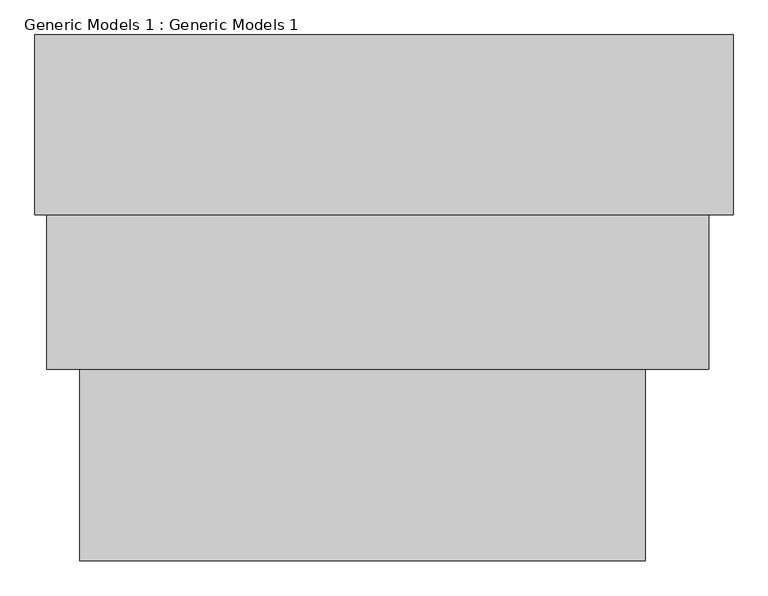
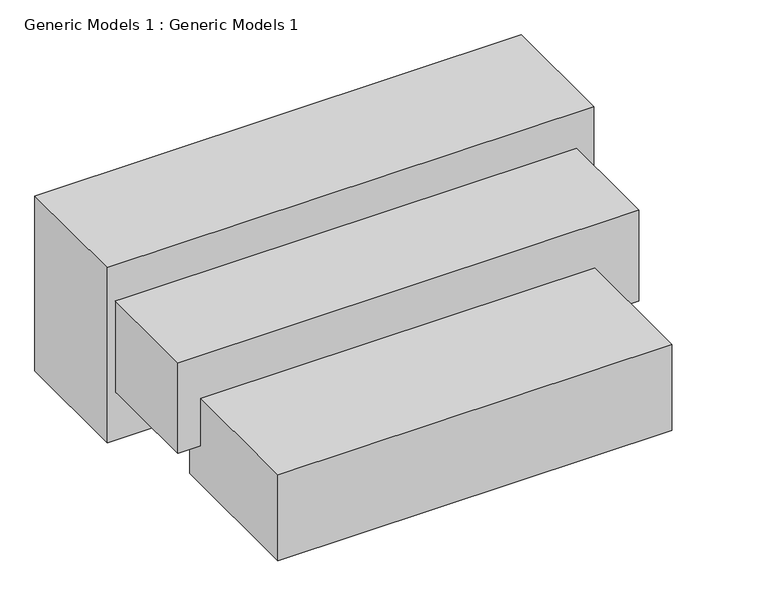
"""IFC4 building model written with IfcOpenShell, lengths in millimetres: proxy geometry, Generic Models 1 : Generic Models 1."""

from ifc_helpers import new_model, si_unit, frame, origin, place, context, project, spatial, polyline, outline, extrude, source, transform, mapped, element, save


def generic_models_1_generic_models_1_22b824c4(model_context):
    return source(origin(), model_context, "Body", "SweptSolid", [
        extrude(outline(polyline([(2976.4110568, 1086.8719151), (2976.4110568, 1471.821948), (3971.3936323, 1471.821948), (3971.3936323, 1086.8719151), (2976.4110568, 1086.8719151)])), frame((0.0, 0.0, -178.9427451), z_axis=(0.0, 0.0, 1.0), x_axis=(1.0, 0.0, 0.0)), (0.0, 0.0, 1.0), 229.7562689),
        extrude(outline(polyline([(2918.2285918, 1423.9390503), (2918.2285918, 1779.7588841), (4083.05, 1779.7588841), (4083.05, 1423.9390503), (2918.2285918, 1423.9390503)])), frame((0.0, 0.0, -76.2), z_axis=(0.0, 0.0, 1.0), x_axis=(1.0, 0.0, 0.0)), (0.0, 0.0, 1.0), 242.6189423),
        extrude(outline(polyline([(2897.395046, 1696.0473527), (2897.395046, 2012.5100722), (4126.0919946, 2012.5100722), (4126.0919946, 1696.0473527), (2897.395046, 1696.0473527)])), frame((0.0, 0.0, -204.7690848), z_axis=(0.0, 0.0, 1.0), x_axis=(1.0, 0.0, 0.0)), (0.0, 0.0, 1.0), 467.5207201),
    ])


if __name__ == "__main__":
    model = new_model("IFC4")
    model_context = context("Model", 3, world=origin())
    ifc_project = project(units=[si_unit("LENGTHUNIT", "METRE", prefix="MILLI")], contexts=[model_context])
    site = spatial("IfcSite", under=ifc_project)
    building = spatial("IfcBuilding", under=site)
    placement = place(None, origin())
    generic_models_1_generic_models_1_shape = generic_models_1_generic_models_1_22b824c4(model_context)
    element("IfcBuildingElementProxy", 1, Name="Generic Models 1 : Generic Models 1", ObjectType="Generic Models 1 : Generic Models 1", at=placement, inside=building, context=model_context, shape_type="MappedRepresentation", body=[
        mapped(generic_models_1_generic_models_1_shape, transform((0.0, 0.0, 0.0), x_axis=(1.0, 0.0, 0.0), y_axis=(0.0, 1.0, 0.0), z_axis=(0.0, 0.0, 1.0))),
    ])
    save(model, "model.ifc")

# Revit data of these elements
# Element 1 (IfcBuildingElementProxy, "Generic Models 1 : Generic Models 1")
#   Materials on its faces: "Door - Panel"
# Materials
#   "Door - Panel": class "Wood", colour RGB 210 159 95, transparency 0, Cost = 0
